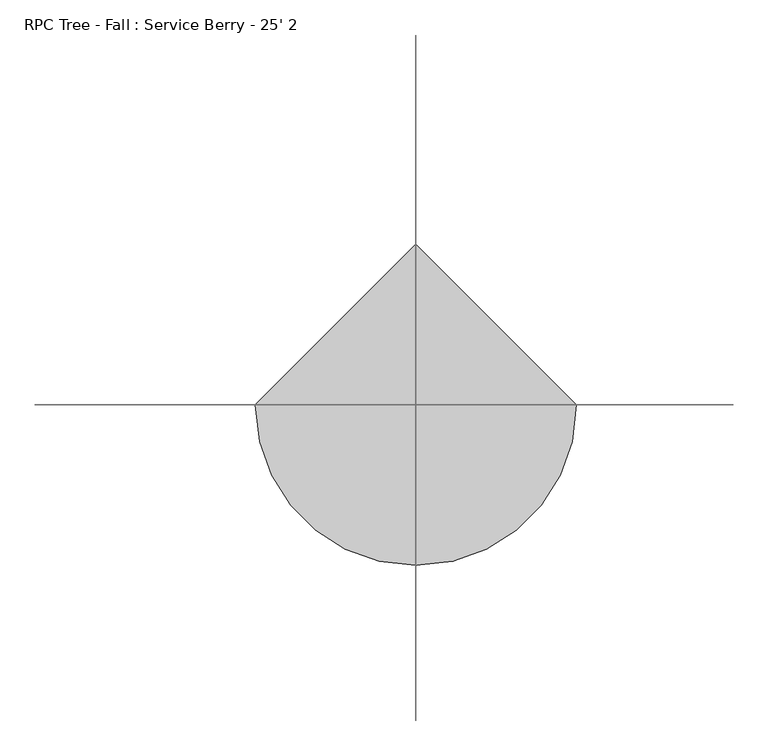
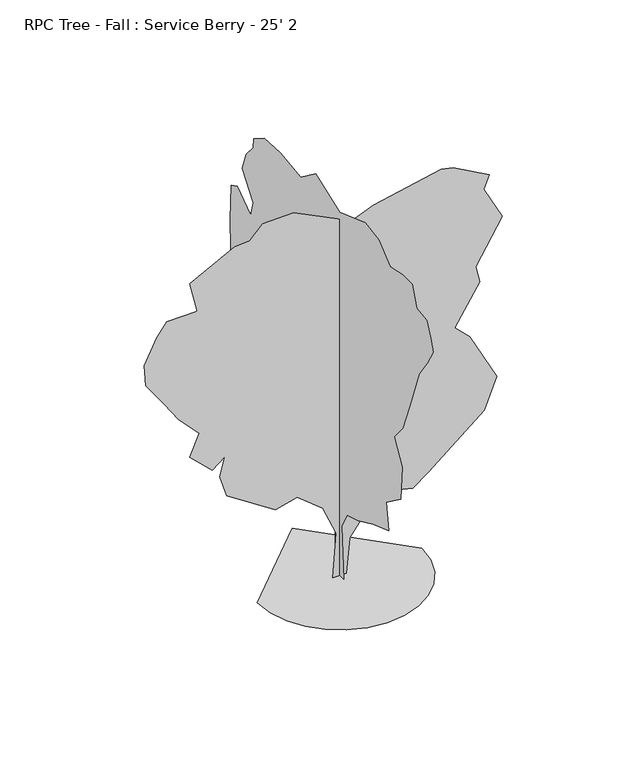
"""IFC4 building model written with IfcOpenShell, lengths in millimetres: geographic element geometry, RPC Tree - Fall : Service Berry - 25' 2."""

from ifc_helpers import new_model, si_unit, origin, place, context, project, spatial, triangles, source, transform, mapped, element, save


def rpc_tree_fall_service_berry_25_2_d25f016d(model_context):
    return source(origin(), model_context, "Body", "Tessellation", [
        triangles([(-1883.0463982, 0.0, 0.1106392), (-1833.2635357, -431.4683584, 0.1106392), (-1691.4858524, -827.7049284, 0.1106392), (-1469.0643997, -1177.3558971, 0.1106392), (-1177.3558971, -1469.0643997, 0.1106392), (-827.7049284, -1691.4858524, 0.1106392), (-431.4683584, -1833.2635357, 0.1106392), (8.23e-05, -1883.0463982, 0.1106392), (431.4683584, -1833.2635357, 0.1106392), (827.7049284, -1691.4858524, 0.1106392), (1177.3558971, -1469.0643997, 0.1106392), (1469.0674519, -1177.3558971, 0.1106392), (1691.4858524, -827.7049284, 0.1106392), (1833.2635357, -431.4683584, 0.1106392), (1883.0463982, 0.0001646, 0.1106392), (-0.0002469, 1883.0463982, 0.1106392), (-2.02e-05, -169.8209752, 0.1767107), (0.0001377, -83.6909853, 1238.6419819), (0.0001596, -307.6617803, 1646.3024185), (0.0001229, -738.4260029, 1769.3774643), (8.44e-05, -1338.415107, 2046.2971893), (3.85e-05, -1938.404211, 2261.6777927), (0.0001247, -1846.0986534, 2892.4362396), (0.0001064, -2415.318124, 3307.8082695), (0.0001962, -2476.8572456, 4123.177977), (0.0002604, -2276.8598602, 4461.6273766), (0.0002989, -2153.7848145, 4661.6369705), (0.0003063, -2507.6265884, 5077.0180115), (0.0003576, -2769.1600433, 5769.3094757), (0.0004337, -3148.0627876, 6786.6398209), (0.0004493, -3461.4576118, 7230.8243362), (0.0004695, -3707.6140984, 7646.2053772), (0.0005154, -3599.9282295, 7923.1158005), (0.000574, -3446.0652374, 8261.5654907), (0.0006272, -3061.469236, 8323.1041763), (0.0007043, -2876.848819, 8784.6318192), (0.0007498, -2495.4866318, 8785.0585373), (0.0007965, -1995.5449093, 8677.494754), (0.0008961, -1539.3665039, 9056.1169922), (0.0009693, -1012.6604267, 9143.9906982), (0.0010469, -0.7067177, 8783.1691177), (0.0012023, 947.0461905, 9138.7485764), (0.001221, 1540.923967, 8701.6961838), (0.0013296, 2353.8308887, 8800.0244843), (0.0014012, 2984.5893356, 8769.2699661), (0.0014195, 3415.3415314, 8492.3293121), (0.0013948, 3431.1911453, 8269.7644089), (0.0013883, 3707.6443291, 7938.5078842), (0.0013553, 3861.5073212, 7507.7347595), (0.0012359, 3417.3835579, 6950.1339111), (0.001205, 3535.3106621, 6573.3406311), (0.0013123, 4053.1043472, 6955.3463837), (0.0013278, 4307.6425896, 6830.835379), (0.0012306, 4338.4273384, 5984.6812134), (0.0010612, 4298.6509872, 4603.5117393), (0.0009225, 3707.6443291, 4030.8844826), (0.0007483, 3153.8234825, 3123.19105), (0.0006249, 2448.8339561, 2793.3885063), (0.0005099, 1717.8083736, 2559.6559708), (0.0004905, 1391.5416607, 2723.2084877), (0.0004255, 1138.4664831, 2430.9055447), (0.0004016, 1246.1583836, 2123.2163315), (0.000365, 1169.2360439, 1892.4525101), (0.0002622, 722.3447897, 1477.0745213), (0.0002515, 377.814475, 1731.7896423), (0.0001768, 172.355686, 1310.8368484), (1.83e-05, 153.6199655, 0.1048395), (-157.3839254, 6.9e-06, 1.33e-05), (-80.7548546, -0.0001217, 1050.4860249), (-386.6810849, -0.0001933, 1763.110841), (-975.7461102, -0.0002234, 2231.9963196), (-1475.2548649, -0.000186, 2101.3896114), (-2587.4964226, -0.0002243, 2830.7205299), (-2748.4671204, -0.0002793, 3350.6326904), (-2633.6491287, -0.0003379, 3799.9378235), (-2916.1376999, -0.0002983, 3571.5209518), (-3433.6296593, -0.0003341, 4061.4558723), (-3217.3742546, -0.0004036, 4565.8079361), (-3679.7858551, -0.0004425, 5061.4427994), (-4018.2352547, -0.0004864, 5553.755191), (-4433.6162956, -0.0005379, 6138.3607864), (-4469.9483803, -0.0005962, 6640.152832), (-4189.7460068, -0.000678, 7223.6916321), (-3956.6962784, -0.0007238, 7522.9442963), (-3258.1563583, -0.0007558, 7534.7092758), (-3433.6296593, -0.0008347, 8261.4125931), (-2402.8822552, -0.000944, 8799.8413559), (-2056.9895599, -0.0009616, 8820.720314), (-1756.7404449, -0.0010107, 9122.9291931), (-1055.3262817, -0.0010437, 9141.9791931), (280.6888264, -0.0010241, 8487.7877289), (766.2938513, -0.0010697, 8692.1560684), (2320.1139061, -0.0011761, 9015.2433243), (2597.0336311, -0.0011809, 8953.7046387), (3423.2052956, -0.0011623, 8495.10298), (3300.675856, -0.0011206, 8190.0593903), (3721.0251984, -0.001043, 7385.3573456), (3116.4246025, -0.0008964, 6377.140979), (3201.9818802, -0.0008533, 5984.3457687), (2631.6832603, -0.0007201, 5075.6768143), (2980.9622314, -0.000694, 4728.7235733), (3594.4114151, -0.0005814, 3559.4812798), (3312.2582886, -0.0004834, 2840.3184906), (2027.8111084, -0.0003014, 1784.5839489), (1666.0138607, -0.000255, 1528.573558), (997.0607975, -0.0002453, 1692.2783913), (643.0633644, -0.0001936, 1388.1706455), (232.6728074, -0.0001098, 835.6723927), (145.7680193, -6.4e-06, 0.0)], [[15, 16, 1], [14, 15, 1], [14, 1, 2], [13, 14, 2], [13, 2, 3], [13, 3, 4], [12, 13, 4], [11, 12, 4], [11, 4, 5], [11, 5, 6], [11, 6, 7], [11, 7, 8], [11, 8, 9], [11, 9, 10], [67, 17, 18], [66, 67, 18], [63, 64, 65], [21, 22, 23], [66, 18, 19], [65, 66, 19], [35, 36, 37], [51, 52, 53], [51, 53, 54], [62, 63, 65], [61, 62, 65], [48, 49, 50], [41, 42, 43], [33, 34, 35], [47, 48, 50], [51, 54, 55], [51, 55, 56], [45, 46, 47], [31, 32, 33], [31, 33, 35], [30, 31, 35], [35, 37, 38], [30, 35, 38], [29, 30, 38], [23, 24, 25], [23, 25, 26], [23, 26, 27], [44, 45, 47], [44, 47, 50], [43, 44, 50], [58, 59, 60], [41, 43, 50], [41, 50, 51], [41, 51, 56], [41, 56, 57], [41, 57, 58], [41, 58, 60], [40, 41, 60], [39, 40, 60], [38, 39, 60], [29, 38, 60], [28, 29, 60], [27, 28, 60], [23, 27, 60], [23, 60, 61], [21, 23, 61], [20, 21, 61], [20, 61, 65], [20, 65, 19], [109, 68, 69], [108, 109, 69], [107, 108, 69], [107, 69, 70], [94, 95, 96], [75, 76, 77], [75, 77, 78], [85, 86, 87], [106, 107, 70], [96, 97, 98], [85, 87, 88], [83, 84, 85], [101, 102, 103], [101, 103, 104], [100, 101, 104], [104, 105, 106], [100, 104, 106], [100, 106, 70], [100, 70, 71], [94, 96, 98], [93, 94, 98], [92, 93, 98], [91, 92, 98], [71, 72, 73], [100, 71, 73], [100, 73, 74], [100, 74, 75], [100, 75, 78], [99, 100, 78], [98, 99, 78], [91, 98, 78], [90, 91, 78], [89, 90, 78], [88, 89, 78], [85, 88, 78], [85, 78, 79], [85, 79, 80], [83, 85, 80], [83, 80, 81], [82, 83, 81]], closed=False),
    ])


if __name__ == "__main__":
    model = new_model("IFC4")
    model_context = context("Model", 3, world=origin())
    ifc_project = project(units=[si_unit("LENGTHUNIT", "METRE", prefix="MILLI")], contexts=[model_context])
    site = spatial("IfcSite", under=ifc_project)
    building = spatial("IfcBuilding", under=site)
    placement = place(None, origin())
    rpc_tree_fall_service_berry_25_2_shape = rpc_tree_fall_service_berry_25_2_d25f016d(model_context)
    element("IfcGeographicElement", 1, ObjectType="RPC Tree - Fall : Service Berry - 25' 2", at=placement, inside=building, context=model_context, shape_type="MappedRepresentation", body=[
        mapped(rpc_tree_fall_service_berry_25_2_shape, transform((0.0, 0.0, 0.0), x_axis=(1.0, 0.0, 0.0), y_axis=(0.0, 1.0, 0.0), z_axis=(0.0, 0.0, 1.0))),
    ])
    save(model, "model.ifc")

# Revit data of these elements
# Type "RPC Tree - Fall : Service Berry - 25' 2"
#   built-in parameter 1005198 = "{2, 15},{39, RPC-16-FVGU-8VG0-7PL0-4000-ST1L-LVER-AU},{1, 0},{1, 0},{2, 13},{1, 8},{5, Color},{1, 0},{1, 0},{3, 0.8},{3, 0.8},{3, 0.8},{1, 8},{7, BBoxMin},{1, 0},{1, 0},{1, 0},{1, 0},{1, 0},{1, 8},{7, BBoxMax},{1, 0},{1, 0},{1, 0},{1, 0},{1, 0},{2, 11},{9, RPCTypeId},{1, 0},{1, 0},{39, RPC-16-FVGU-8VG0-7PL0-4000-ST1L-LVER-AU},{1, 6},{14, RPCPlantHeight},{1, 0},{1, 0},{2, 25},{2, 11},{7, keyword},{1, 0},{1, 0},{39, :RPCs:Fall Trees [General]:Geometry:RPC},{2, 11},{8, category},{1, 0},{1, 0},{20, Fall Trees [General]},{2, 11},{12, LocalizedUID},{1, 0},{1, 0},{20, Service Berry [Fall]},{2, 14},{6, Height},{1, 0},{1, 0},{2, 25},{1, 2},{16, Cast Reflections},{1, 0},{1, 0},{1, 0},{1, 2},{12, Cast Shadows},{1, 0},{1, 0},{1, 1},{1, 2},{9, Lock View},{1, 0},{1, 0},{1, 0},{1, 4},{5, ViewC},{1, 0},{1, 0},{1, 0},{21, assetlibrary_base.fbx},{1, 5},"
#   built-in parameter 1005195 = "RPC-16-FVGU-8VG0-7PL0-4000-ST1L-LVER-AU"
#   Type Comments = "Service Berry"
#   Assembly Code = "G2050500"
#   Height = 30' - 0"
#   Default Elevation = 0
